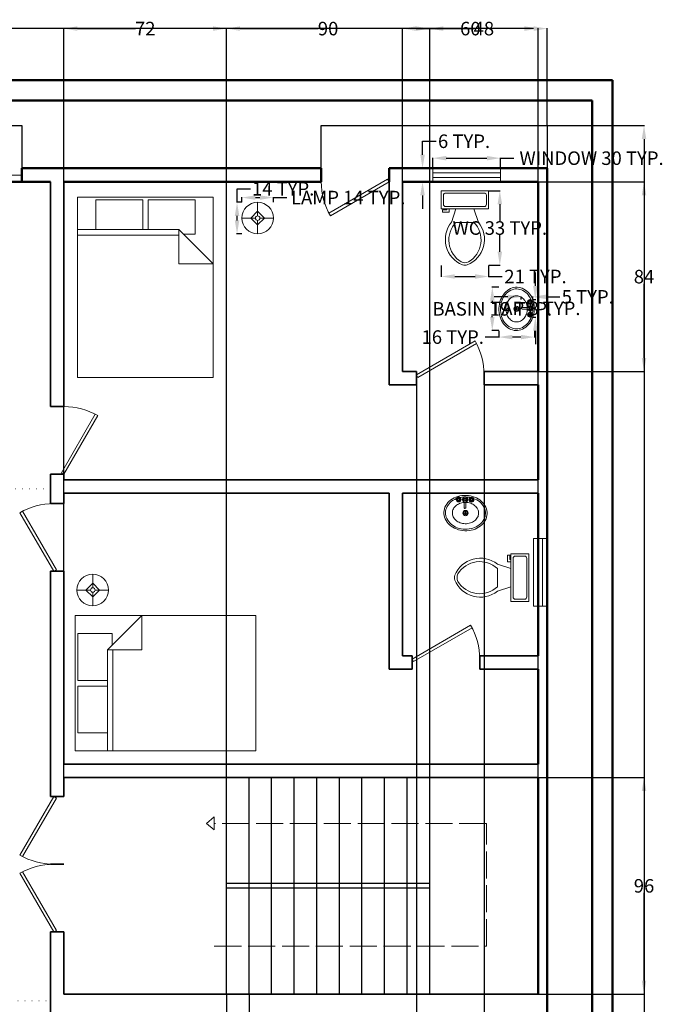
# Model space of a CAD drawing. Units: inches. Extents: x 910 to 1553, y 598 to 1516.
# Tile 6 of 6: x 1268 to 1553, y 1079 to 1516. Entities that reach past the tile are written whole.
import ezdxf

# ---------------------------------------------------------------- set-up
doc = ezdxf.new("R2010")
doc.units = ezdxf.units.IN
doc.header["$MEASUREMENT"] = 0
doc.linetypes.add('ACAD_ISO02W100', pattern=[15, 12, -3])
doc.linetypes.add('ACAD_ISO07W100', pattern=[3, 0, -3])
for name, color, linetype, lineweight in [('A-ANNO-DIMS', 2, 'Continuous', 18), ('A-ANNO-SYMB', 7, 'Continuous', 13), ('A-FLOR-BALC', 8, 'Continuous', 25), ('A-FLOR-OVHD', 8, 'ACAD_ISO07W100', 13), ('A-FLOR-STRS', 7, 'Continuous', 25), ('A-FLOR-STRS-PATH', 7, 'ACAD_ISO02W100', 13), ('doors', 2, 'Continuous', 18), ('furniture', 11, 'Continuous', 18), ('Inner wall', 230, 'Continuous', 35), ('outer wall', 231, 'Continuous', 50), ('sanitory', 141, 'Continuous', 18), ('windows', 6, 'Continuous', 18)]:
    doc.layers.add(name, color=color, linetype=linetype, lineweight=lineweight)
doc.styles.get("Standard").update_dxf_attribs({"font": 'arial.ttf'})
doc.dimstyles.get("Standard").update_dxf_attribs({"dimtxt": 6, "dimasz": 6, "dimexe": 0.18, "dimexo": 0.0625, "dimgap": 0.09, "dimtad": 0, "dimtih": 1, "dimtoh": 1, "dimdec": 0, "dimzin": 0, "dimdsep": 46, "dimlunit": 3, "dimtxsty": 'Standard', "dimcen": 0.09, "dimadec": 0, "dimazin": 0, "dimtfac": 1, "dimtdec": 0, "dimtofl": 0, "dimtmove": 0, "dimatfit": 3, "dimfxl": 1, "dimtolj": 1, "dimtzin": 0, "dimarcsym": 0})

# ---------------------------------------------------------------- blocks, each defined once
blk = doc.blocks.new('*U2')
for p, q in [((0, 0), (0, -6)), ((40, 0), (40, -6))]:
    blk.add_line(p, q)
blk.add_lwpolyline([(0, 0), (34.64, 20), (35.52, 18.48), (0.87, -1.52)], close=True)
blk.add_arc((0, 0), 40, 0, 30)
blk = doc.blocks.new('*U4')
for p, q in [((0, 0), (0, 6)), ((40, 0), (40, 6))]:
    blk.add_line(p, q)
blk.add_lwpolyline([(0, 0), (34.64, -20), (35.52, -18.48), (0.87, 1.52)], close=True)
blk.add_arc((0, 0), 40, 330, 0)
blk = doc.blocks.new('*U5')
for p, q in [((0, 0), (0, -6)), ((-40, 0), (-40, -6))]:
    blk.add_line(p, q)
blk.add_lwpolyline([(0, 0), (-34.64, 20), (-35.52, 18.48), (-0.88, -1.52)], close=True)
blk.add_arc((0, 0), 40, 150, 180)
blk = doc.blocks.new('*U7')
for p, q in [((-40, 0), (-40, 6)), ((0, 0), (0, 6))]:
    blk.add_line(p, q)
blk.add_lwpolyline([(0, 0), (-34.64, -20), (-35.52, -18.48), (-0.88, 1.52)], close=True)
blk.add_arc((0, 0), 40, 180, 210)
blk = doc.blocks.new('Bed - Queen')
for p, q in [((0, -80.00003), (0, 0)), ((0, 0), (59.99999, 0)), ((59.99999, 0), (59.99999, -80.00003)), ((7.99999, -1.2), (28.79998, -1.2)), ((7.99999, -14.4), (7.99999, -1.2)), ((28.79998, -1.2), (28.79998, -14.4)), ((31.19999, -1.2), (51.99999, -1.2)), ((31.19999, -14.4), (31.19999, -1.2)), ((51.99999, -1.2), (51.99999, -16.4)), ((0, -14.4), (44.8, -14.4)), ((44.8, -16.8), (0, -16.8)), ((59.99999, -29.6), (44.8, -14.4)), ((44.8, -14.4), (44.8, -29.6)), ((51.99999, -16.4), (46.79936, -16.4)), ((44.8, -29.6), (59.99999, -29.6)), ((59.99999, -80.00003), (0, -80.00003))]:
    blk.add_line(p, q)
blk = doc.blocks.new('Lamp - Table')
for p, q in [((0, 7), (0, 1)), ((-1, 0), (-7, 0)), ((0, 3), (-3, 0)), ((-3, 0), (0, -3)), ((3, 0), (0, 3)), ((0, -3), (3, 0)), ((1, 0), (7, 0)), ((0, -1), (0, -7))]:
    blk.add_line(p, q)
for radius in [7, 1]:
    blk.add_circle((0, 0), radius)
blk = doc.blocks.new('Toilet - top')
for p, q in [((9.5, -6), (9.5, -2)), ((-10, -8.5), (-8, -8.5)), ((-10, -9.5), (-10, -8.5)), ((-8, -8.5), (-8, -8)), ((-7, -8), (-7, -9.5)), ((-4, -8), (-6, -14)), ((4, -8), (6, -14)), ((-7, -9.5), (-10, -9.5)), ((4, -14), (-4, -14))]:
    blk.add_line(p, q)
blk.add_lwpolyline([(10.5, -8), (10.5, 0), (-10.5, 0), (-10.5, -8)], close=True)
for points in [[(-9.5, -2), (-9.5, -6)], [(8.5, -1), (-8.5, -1)], [(-8.5, -7), (8.5, -7)]]:
    blk.add_lwpolyline(points)
for centre, radius, start, end in [((-8.62, -1.88), 0.884, 81.8699, 188.1301), ((8.62, -1.88), 0.884, 351.8699, 98.1301), ((-8.62, -6.12), 0.884, 171.8699, 278.1301), ((8.62, -6.12), 0.884, 261.8699, 8.1301), ((3.52, -21.58), 12.17, 141.4691, 247.9714), ((4.2, -21.82), 11.33, 136.3677, 238.9468), ((-3.52, -21.58), 12.17, 292.0284, 38.5307), ((-4.2, -21.82), 11.33, 301.053, 43.6321), ((0, -27.88), 4, 245.7318, 294.2682), ((0, -29), 4, 254.8605, 285.1395)]:
    blk.add_arc(centre, radius, start, end)
blk = doc.blocks.new('Faucet - Bathroom top')
for p, q in [((-4.107, 0.125), (-4.375, 0.125)), ((-3.75, 0.4788), (-3.75, 0.75)), ((-3.5, 0.482), (-3.5, 0.75)), ((-3.1461, 0.125), (-2.875, 0.125)), ((3.143, 0.125), (2.875, 0.125)), ((3.5, 0.4788), (3.5, 0.75)), ((3.75, 0.482), (3.75, 0.75)), ((4.1039, 0.125), (4.375, 0.125)), ((-4.1039, -0.125), (-4.375, -0.125)), ((-3.75, -0.4821), (-3.75, -0.75)), ((-3.5, -0.4789), (-3.5, -0.75)), ((-3.143, -0.125), (-2.875, -0.125)), ((-0.5, -0.8639), (-0.5, -4.5)), ((0.5, -4.5), (0.5, -0.8631)), ((3.1461, -0.125), (2.875, -0.125)), ((3.5, -0.4821), (3.5, -0.75)), ((3.75, -0.4789), (3.75, -0.75)), ((4.107, -0.125), (4.375, -0.125))]:
    blk.add_line(p, q)
for centre, radius in [((-3.625, 0), 1.375), ((-4.625, 0), 0.2795), ((-3.625, 0), 0.5), ((-3.625, 1), 0.2795), ((-2.625, 0), 0.2795), ((0, 0), 0.5), ((3.625, 0), 1.375), ((2.625, 0), 0.2795), ((3.625, 0), 0.5), ((3.625, 1), 0.2795), ((4.625, 0), 0.2795), ((-3.625, -1), 0.2795), ((3.625, -1), 0.2795)]:
    blk.add_circle(centre, radius)
for centre, radius, start, end in [((-3.625, 0), 1, 105.2407, 164.2093), ((-3.625, 0), 1, 16.44125, 74.07887), ((0, 0), 1.5, 289.6514, 250.3603), ((0, 0), 1, 300.3431, 239.7554), ((3.625, 0), 1, 106.12, 164.0884), ((3.625, 0), 1, 16.23422, 73.90469), ((-3.625, 0), 1, 196.2342, 253.9047), ((-3.625, 0), 1, 286.12, 344.0884), ((0, -4.5), 0.5, 180, 0), ((3.625, 0), 1, 196.4413, 254.0789), ((3.625, 0), 1, 285.2407, 344.2093)]:
    blk.add_arc(centre, radius, start, end)
blk = doc.blocks.new('Sink - Oval top')
for p, q in [((-1, 0), (1, 0)), ((0, 1), (0, -1))]:
    blk.add_line(p, q)
for points in [[(-12.23, 0.39, 0.117634), (-11.46, -3.36, 0.104469), (-8.88, -6.8, 0.090016), (-5.08, -9.07, 0.08192), (-0.32, -10.02, 0.08192), (4.49, -9.38, 0.090016), (8.42, -7.36, 0.104469), (11.22, -4.09, 0.117634), (12.23, -0.39, 0.117634), (11.46, 3.36, 0.104469), (8.88, 6.8, 0.090016), (5.08, 9.07, 0.08192), (0.32, 10.02, 0.08192), (-4.49, 9.38, 0.090016), (-8.42, 7.36, 0.104469), (-11.22, 4.09, 0.117634)], [(-11.29, 0.16, 0.118622), (-10.52, -3.25, 0.104678), (-8.07, -6.36, 0.089562), (-4.54, -8.37, 0.081185), (-0.13, -9.15, 0.081185), (4.3, -8.49, 0.089562), (7.89, -6.58, 0.104678), (10.42, -3.55, 0.118622), (11.29, -0.16, 0.118622), (10.52, 3.25, 0.104678), (8.07, 6.36, 0.089562), (4.54, 8.37, 0.081185), (0.13, 9.15, 0.081185), (-4.3, 8.49, 0.089562), (-7.89, 6.58, 0.104678), (-10.42, 3.55, 0.118622)], [(-7.42, 0.08, 0.118283), (-6.91, -2.17, 0.104607), (-5.29, -4.21, 0.089718), (-2.97, -5.53, 0.081436), (-0.07, -6.04, 0.081436), (2.84, -5.59, 0.089718), (5.2, -4.33, 0.104607), (6.86, -2.32, 0.118283), (7.42, -0.08, 0.118283), (6.91, 2.17, 0.104607), (5.29, 4.21, 0.089718), (2.97, 5.53, 0.081436), (0.07, 6.04, 0.081436), (-2.84, 5.59, 0.089718), (-5.2, 4.33, 0.104607), (-6.86, 2.32, 0.118283)]]:
    blk.add_lwpolyline(points, format="xyb", close=True)
for radius in [1.5, 1]:
    blk.add_circle((0, 0), radius)
blk = doc.blocks.new('WIN-30X6')
for p, q in [((0, 6), (30, 6)), ((0, 0), (0, 6)), ((30, 6), (30, 0)), ((0, 4), (30, 4)), ((30, 2), (0, 2)), ((30, 0), (0, 0))]:
    blk.add_line(p, q)
blk = doc.blocks.new('VERANDA-EDGE-SHALLOW')
for p, q in [((0, 0), (0, 18.99)), ((0, 18.99), (100, 18.99)), ((100, 18.99), (100, 0))]:
    blk.add_line(p, q)
blk = doc.blocks.new('*D23')
at = {"layer": 'A-ANNO-DIMS', "color": 0, "lineweight": -2, "transparency": 16777216}
for p, q in [((1366.48, 1434.97), (1366.48, 1437.19)), ((1372.48, 1437.01), (1374.48, 1437.01)), ((1380.48, 1434.97), (1380.48, 1437.19)), ((1380.48, 1437.01), (1386.48, 1437.01))]:
    blk.add_line(p, q, dxfattribs=at)
for points in [[(1372.48, 1438.01), (1372.48, 1436.01), (1366.48, 1437.01)], [(1374.48, 1438.01), (1374.48, 1436.01), (1380.48, 1437.01)]]:
    blk.add_solid(points, dxfattribs=at)
at = {"layer": 'Defpoints', "color": 0, "lineweight": -2, "transparency": 16777216}
for p in [(1380.48, 1437.01), (1366.48, 1434.91), (1380.48, 1434.91)]:
    blk.add_point(p, dxfattribs=at)
at = {"layer": 'A-ANNO-DIMS', "color": 0, "transparency": 16777216, "insert": (1413.62, 1437.01), "char_height": 6, "attachment_point": 5}
blk.add_mtext('\\A1;LAMP 14 TYP.', dxfattribs=at)
blk = doc.blocks.new('*D24')
at = {"layer": 'A-ANNO-DIMS', "color": 0, "lineweight": -2, "transparency": 16777216}
for p, q in [((1364.38, 1434.91), (1364.38, 1440.91)), ((1364.38, 1440.91), (1370.38, 1440.91)), ((1366.42, 1434.91), (1364.2, 1434.91)), ((1364.38, 1426.91), (1364.38, 1428.91)), ((1366.42, 1420.91), (1364.2, 1420.91))]:
    blk.add_line(p, q, dxfattribs=at)
for points in [[(1363.38, 1428.91), (1365.38, 1428.91), (1364.38, 1434.91)], [(1363.38, 1426.91), (1365.38, 1426.91), (1364.38, 1420.91)]]:
    blk.add_solid(points, dxfattribs=at)
at = {"layer": 'Defpoints', "color": 0, "lineweight": -2, "transparency": 16777216}
for p in [(1364.38, 1434.91), (1366.48, 1434.91), (1366.48, 1420.91)]:
    blk.add_point(p, dxfattribs=at)
at = {"layer": 'A-ANNO-DIMS', "color": 0, "transparency": 16777216, "insert": (1384.79, 1440.91), "char_height": 6, "attachment_point": 5}
blk.add_mtext('\\A1;14 TYP.', dxfattribs=at)
blk = doc.blocks.new('*D29')
at = {"layer": 'A-ANNO-DIMS', "color": 0, "lineweight": -2, "transparency": 16777216}
for p, q in [((1475.88, 1440.03), (1480.95, 1440.03)), ((1480.77, 1434.03), (1480.77, 1426.7)), ((1480.77, 1412.99), (1480.77, 1420.32)), ((1475.88, 1406.99), (1480.95, 1406.99))]:
    blk.add_line(p, q, dxfattribs=at)
for points in [[(1479.77, 1434.03), (1481.77, 1434.03), (1480.77, 1440.03)], [(1479.77, 1412.99), (1481.77, 1412.99), (1480.77, 1406.99)]]:
    blk.add_solid(points, dxfattribs=at)
at = {"layer": 'Defpoints', "color": 0, "lineweight": -2, "transparency": 16777216}
for p in [(1475.81, 1440.03), (1480.77, 1440.03), (1475.81, 1406.99)]:
    blk.add_point(p, dxfattribs=at)
at = {"layer": 'A-ANNO-DIMS', "color": 0, "transparency": 16777216, "insert": (1480.77, 1423.51), "char_height": 6, "attachment_point": 5}
blk.add_mtext('\\A1;WC 33 TYP.', dxfattribs=at)
blk = doc.blocks.new('*D30')
at = {"layer": 'A-ANNO-DIMS', "color": 0, "lineweight": -2, "transparency": 16777216}
for p, q in [((1454.81, 1406.92), (1454.81, 1401.85)), ((1475.81, 1406.92), (1475.81, 1401.85)), ((1460.81, 1402.03), (1469.81, 1402.03)), ((1475.81, 1402.03), (1481.81, 1402.03))]:
    blk.add_line(p, q, dxfattribs=at)
for points in [[(1460.81, 1403.03), (1460.81, 1401.03), (1454.81, 1402.03)], [(1469.81, 1403.03), (1469.81, 1401.03), (1475.81, 1402.03)]]:
    blk.add_solid(points, dxfattribs=at)
at = {"layer": 'Defpoints', "color": 0, "lineweight": -2, "transparency": 16777216}
for p in [(1454.81, 1406.99), (1475.81, 1406.99), (1475.81, 1402.03)]:
    blk.add_point(p, dxfattribs=at)
at = {"layer": 'A-ANNO-DIMS', "color": 0, "transparency": 16777216, "insert": (1496.56, 1402.03), "char_height": 6, "attachment_point": 5}
blk.add_mtext('\\A1;21 TYP.', dxfattribs=at)
blk = doc.blocks.new('*D31')
at = {"layer": 'A-ANNO-DIMS', "color": 0, "lineweight": -2, "transparency": 16777216}
for p, q in [((1480.26, 1397.29), (1477.25, 1397.29)), ((1477.43, 1391.29), (1477.43, 1390.87)), ((1477.43, 1384.06), (1477.43, 1384.48)), ((1480.26, 1378.06), (1477.25, 1378.06))]:
    blk.add_line(p, q, dxfattribs=at)
for points in [[(1476.43, 1391.29), (1478.43, 1391.29), (1477.43, 1397.29)], [(1476.43, 1384.06), (1478.43, 1384.06), (1477.43, 1378.06)]]:
    blk.add_solid(points, dxfattribs=at)
at = {"layer": 'Defpoints', "color": 0, "lineweight": -2, "transparency": 16777216}
for p in [(1477.43, 1397.29), (1480.32, 1397.29), (1480.32, 1378.06)]:
    blk.add_point(p, dxfattribs=at)
at = {"layer": 'A-ANNO-DIMS', "color": 0, "transparency": 16777216, "insert": (1477.43, 1387.68), "char_height": 6, "attachment_point": 5}
blk.add_mtext('\\A1;BASIN 19 TYP.', dxfattribs=at)
blk = doc.blocks.new('*D32')
at = {"layer": 'A-ANNO-DIMS', "color": 0, "lineweight": -2, "transparency": 16777216}
for p, q in [((1480.32, 1375.18), (1474.32, 1375.18)), ((1480.32, 1378), (1480.32, 1375)), ((1490.09, 1375.18), (1486.32, 1375.18)), ((1496.09, 1378), (1496.09, 1375))]:
    blk.add_line(p, q, dxfattribs=at)
for points in [[(1486.32, 1376.18), (1486.32, 1374.18), (1480.32, 1375.18)], [(1490.09, 1376.18), (1490.09, 1374.18), (1496.09, 1375.18)]]:
    blk.add_solid(points, dxfattribs=at)
at = {"layer": 'Defpoints', "color": 0, "lineweight": -2, "transparency": 16777216}
for p in [(1480.32, 1378.06), (1480.32, 1375.18), (1496.09, 1378.06)]:
    blk.add_point(p, dxfattribs=at)
at = {"layer": 'A-ANNO-DIMS', "color": 0, "transparency": 16777216, "insert": (1459.91, 1375.18), "char_height": 6, "attachment_point": 5}
blk.add_mtext('\\A1;16 TYP.', dxfattribs=at)
blk = doc.blocks.new('*D35')
at = {"layer": 'A-ANNO-DIMS', "color": 0, "lineweight": -2, "transparency": 16777216}
for p, q in [((1496.52, 1397.84), (1496.52, 1403.84)), ((1495.41, 1391.84), (1496.7, 1391.84)), ((1495.41, 1384), (1496.7, 1384)), ((1496.52, 1378), (1496.52, 1372))]:
    blk.add_line(p, q, dxfattribs=at)
for points in [[(1495.52, 1397.84), (1497.52, 1397.84), (1496.52, 1391.84)], [(1495.52, 1378), (1497.52, 1378), (1496.52, 1384)]]:
    blk.add_solid(points, dxfattribs=at)
at = {"layer": 'Defpoints', "color": 0, "lineweight": -2, "transparency": 16777216}
for p in [(1495.35, 1391.84), (1495.35, 1384), (1496.52, 1384)]:
    blk.add_point(p, dxfattribs=at)
at = {"layer": 'A-ANNO-DIMS', "color": 0, "transparency": 16777216, "insert": (1496.52, 1387.92), "char_height": 6, "attachment_point": 5}
blk.add_mtext('\\A1;TAP 8 TYP.', dxfattribs=at)
blk = doc.blocks.new('*D36')
at = {"layer": 'A-ANNO-DIMS', "color": 0, "lineweight": -2, "transparency": 16777216}
for p, q in [((1484.26, 1393.01), (1478.26, 1393.01)), ((1490.26, 1391.9), (1490.26, 1393.19)), ((1495.35, 1391.9), (1495.35, 1393.19)), ((1501.35, 1393.01), (1507.35, 1393.01))]:
    blk.add_line(p, q, dxfattribs=at)
for points in [[(1484.26, 1394.01), (1484.26, 1392.01), (1490.26, 1393.01)], [(1501.35, 1394.01), (1501.35, 1392.01), (1495.35, 1393.01)]]:
    blk.add_solid(points, dxfattribs=at)
at = {"layer": 'Defpoints', "color": 0, "lineweight": -2, "transparency": 16777216}
for p in [(1495.35, 1393.01), (1490.26, 1391.84), (1495.35, 1391.84)]:
    blk.add_point(p, dxfattribs=at)
at = {"layer": 'A-ANNO-DIMS', "color": 0, "transparency": 16777216, "insert": (1519.71, 1393.01), "char_height": 6, "attachment_point": 5}
blk.add_mtext('\\A1;5 TYP.', dxfattribs=at)
blk = doc.blocks.new('*D39')
at = {"layer": 'A-ANNO-DIMS', "color": 0, "lineweight": -2, "transparency": 16777216}
for p, q in [((1451.04, 1450.03), (1451.04, 1454.65)), ((1457.04, 1454.47), (1475.04, 1454.47)), ((1481.04, 1450.03), (1481.04, 1454.65)), ((1481.04, 1454.47), (1487.04, 1454.47))]:
    blk.add_line(p, q, dxfattribs=at)
for points in [[(1457.04, 1455.47), (1457.04, 1453.47), (1451.04, 1454.47)], [(1475.04, 1455.47), (1475.04, 1453.47), (1481.04, 1454.47)]]:
    blk.add_solid(points, dxfattribs=at)
at = {"layer": 'Defpoints', "color": 0, "lineweight": -2, "transparency": 16777216}
for p in [(1481.04, 1454.47), (1451.04, 1449.97), (1481.04, 1449.97)]:
    blk.add_point(p, dxfattribs=at)
at = {"layer": 'A-ANNO-DIMS', "color": 0, "transparency": 16777216, "insert": (1521.41, 1454.47), "char_height": 6, "attachment_point": 5}
blk.add_mtext('\\A1;WINDOW 30 TYP.', dxfattribs=at)
blk = doc.blocks.new('*D40')
at = {"layer": 'A-ANNO-DIMS', "color": 0, "lineweight": -2, "transparency": 16777216}
for p, q in [((1446.54, 1455.97), (1446.54, 1461.97)), ((1446.54, 1461.97), (1452.54, 1461.97)), ((1450.98, 1449.97), (1446.36, 1449.97)), ((1450.98, 1443.97), (1446.36, 1443.97)), ((1446.54, 1437.97), (1446.54, 1431.97))]:
    blk.add_line(p, q, dxfattribs=at)
for points in [[(1445.54, 1455.97), (1447.54, 1455.97), (1446.54, 1449.97)], [(1445.54, 1437.97), (1447.54, 1437.97), (1446.54, 1443.97)]]:
    blk.add_solid(points, dxfattribs=at)
at = {"layer": 'Defpoints', "color": 0, "lineweight": -2, "transparency": 16777216}
for p in [(1446.54, 1449.97), (1451.04, 1449.97), (1451.04, 1443.97)]:
    blk.add_point(p, dxfattribs=at)
at = {"layer": 'A-ANNO-DIMS', "color": 0, "transparency": 16777216, "insert": (1464.92, 1461.97), "char_height": 6, "attachment_point": 5}
blk.add_mtext('\\A1;6 TYP.', dxfattribs=at)
blk = doc.blocks.new('*D55')
at = {"layer": 'A-ANNO-DIMS', "color": 0, "lineweight": -2, "transparency": 16777216}
for p, q in [((959.7, 1469.02), (959.7, 1512.08)), ((965.7, 1511.9), (1224.01, 1511.9)), ((1495.7, 1511.9), (1237.39, 1511.9)), ((1501.7, 1469.02), (1501.7, 1512.08))]:
    blk.add_line(p, q, dxfattribs=at)
for points in [[(965.7, 1512.9), (965.7, 1510.9), (959.7, 1511.9)], [(1495.7, 1512.9), (1495.7, 1510.9), (1501.7, 1511.9)]]:
    blk.add_solid(points, dxfattribs=at)
at = {"layer": 'Defpoints', "color": 0, "lineweight": -2, "transparency": 16777216}
for p in [(1501.7, 1511.9), (959.7, 1468.95), (1501.7, 1468.95)]:
    blk.add_point(p, dxfattribs=at)
at = {"layer": 'A-ANNO-DIMS', "color": 0, "transparency": 16777216, "insert": (1230.7, 1511.9), "char_height": 6, "attachment_point": 5}
blk.add_mtext('\\A1;542', dxfattribs=at)
blk = doc.blocks.new('*D56')
at = {"layer": 'A-ANNO-DIMS', "color": 0, "lineweight": -2, "transparency": 16777216}
for p, q in [((1501.76, 1468.95), (1544.83, 1468.95)), ((1544.65, 1462.95), (1544.65, 1060.13)), ((1544.65, 650.99), (1544.65, 1053.82)), ((1501.76, 644.99), (1544.83, 644.99))]:
    blk.add_line(p, q, dxfattribs=at)
for points in [[(1543.65, 1462.95), (1545.65, 1462.95), (1544.65, 1468.95)], [(1543.65, 650.99), (1545.65, 650.99), (1544.65, 644.99)]]:
    blk.add_solid(points, dxfattribs=at)
at = {"layer": 'Defpoints', "color": 0, "lineweight": -2, "transparency": 16777216}
for p in [(1501.7, 1468.95), (1544.65, 1468.95), (1501.7, 644.99)]:
    blk.add_point(p, dxfattribs=at)
at = {"layer": 'A-ANNO-DIMS', "color": 0, "transparency": 16777216, "insert": (1544.65, 1056.97), "char_height": 6, "attachment_point": 5}
blk.add_mtext('\\A1;824', dxfattribs=at)
blk = doc.blocks.new('*D71')
at = {"layer": 'A-ANNO-DIMS', "color": 0, "lineweight": -2, "transparency": 16777216}
for p, q in [((1437.7, 1444.03), (1437.7, 1512.08)), ((1443.7, 1511.9), (1463.31, 1511.9)), ((1491.7, 1511.9), (1472.09, 1511.9)), ((1497.7, 1444.03), (1497.7, 1512.08))]:
    blk.add_line(p, q, dxfattribs=at)
for points in [[(1443.7, 1512.9), (1443.7, 1510.9), (1437.7, 1511.9)], [(1491.7, 1512.9), (1491.7, 1510.9), (1497.7, 1511.9)]]:
    blk.add_solid(points, dxfattribs=at)
at = {"layer": 'Defpoints', "color": 0, "lineweight": -2, "transparency": 16777216}
for p in [(1497.7, 1511.9), (1437.7, 1443.97), (1497.7, 1443.97)]:
    blk.add_point(p, dxfattribs=at)
at = {"layer": 'A-ANNO-DIMS', "color": 0, "transparency": 16777216, "insert": (1467.7, 1511.9), "char_height": 6, "attachment_point": 5}
blk.add_mtext('\\A1;60', dxfattribs=at)
blk = doc.blocks.new('*D72')
at = {"layer": 'A-ANNO-DIMS', "color": 0, "lineweight": -2, "transparency": 16777216}
for p, q in [((1497.76, 1443.97), (1544.83, 1443.97)), ((1544.65, 1437.97), (1544.65, 1405.12)), ((1544.65, 1365.97), (1544.65, 1398.82)), ((1497.76, 1359.97), (1544.83, 1359.97))]:
    blk.add_line(p, q, dxfattribs=at)
for points in [[(1543.65, 1437.97), (1545.65, 1437.97), (1544.65, 1443.97)], [(1543.65, 1365.97), (1545.65, 1365.97), (1544.65, 1359.97)]]:
    blk.add_solid(points, dxfattribs=at)
at = {"layer": 'Defpoints', "color": 0, "lineweight": -2, "transparency": 16777216}
for p in [(1497.7, 1443.97), (1544.65, 1443.97), (1497.7, 1359.97)]:
    blk.add_point(p, dxfattribs=at)
at = {"layer": 'A-ANNO-DIMS', "color": 0, "transparency": 16777216, "insert": (1544.65, 1401.97), "char_height": 6, "attachment_point": 5}
blk.add_mtext('\\A1;84', dxfattribs=at)
blk = doc.blocks.new('*D73')
at = {"layer": 'A-ANNO-DIMS', "color": 0, "lineweight": -2, "transparency": 16777216}
for p, q in [((1443.82, 1359.91), (1443.82, 601.86)), ((1473.82, 1359.91), (1473.82, 601.86)), ((1449.82, 602.04), (1454.45, 602.04)), ((1467.82, 602.04), (1463.2, 602.04))]:
    blk.add_line(p, q, dxfattribs=at)
for points in [[(1449.82, 603.04), (1449.82, 601.04), (1443.82, 602.04)], [(1467.82, 603.04), (1467.82, 601.04), (1473.82, 602.04)]]:
    blk.add_solid(points, dxfattribs=at)
at = {"layer": 'Defpoints', "color": 0, "lineweight": -2, "transparency": 16777216}
for p in [(1443.82, 1359.97), (1473.82, 1359.97), (1473.82, 602.04)]:
    blk.add_point(p, dxfattribs=at)
at = {"layer": 'A-ANNO-DIMS', "color": 0, "transparency": 16777216, "insert": (1458.82, 602.04), "char_height": 6, "attachment_point": 5}
blk.add_mtext('\\A1;30', dxfattribs=at)
blk = doc.blocks.new('*D77')
at = {"layer": 'A-ANNO-DIMS', "color": 0, "lineweight": -2, "transparency": 16777216}
for p, q in [((1287.7, 1180.03), (1287.7, 1512.08)), ((1293.7, 1511.9), (1319.37, 1511.9)), ((1353.7, 1511.9), (1328.03, 1511.9)), ((1359.7, 1180.03), (1359.7, 1512.08))]:
    blk.add_line(p, q, dxfattribs=at)
for points in [[(1293.7, 1512.9), (1293.7, 1510.9), (1287.7, 1511.9)], [(1353.7, 1512.9), (1353.7, 1510.9), (1359.7, 1511.9)]]:
    blk.add_solid(points, dxfattribs=at)
at = {"layer": 'Defpoints', "color": 0, "lineweight": -2, "transparency": 16777216}
for p in [(1359.7, 1511.9), (1287.7, 1179.97), (1359.7, 1179.97)]:
    blk.add_point(p, dxfattribs=at)
at = {"layer": 'A-ANNO-DIMS', "color": 0, "transparency": 16777216, "insert": (1323.7, 1511.9), "char_height": 6, "attachment_point": 5}
blk.add_mtext('\\A1;72', dxfattribs=at)
blk = doc.blocks.new('*D78')
at = {"layer": 'A-ANNO-DIMS', "color": 0, "lineweight": -2, "transparency": 16777216}
for p, q in [((1359.7, 1180.03), (1359.7, 1512.08)), ((1365.7, 1511.9), (1400.32, 1511.9)), ((1443.7, 1511.9), (1409.08, 1511.9)), ((1449.7, 1180.03), (1449.7, 1512.08))]:
    blk.add_line(p, q, dxfattribs=at)
for points in [[(1365.7, 1512.9), (1365.7, 1510.9), (1359.7, 1511.9)], [(1443.7, 1512.9), (1443.7, 1510.9), (1449.7, 1511.9)]]:
    blk.add_solid(points, dxfattribs=at)
at = {"layer": 'Defpoints', "color": 0, "lineweight": -2, "transparency": 16777216}
for p in [(1449.7, 1511.9), (1359.7, 1179.97), (1449.7, 1179.97)]:
    blk.add_point(p, dxfattribs=at)
at = {"layer": 'A-ANNO-DIMS', "color": 0, "transparency": 16777216, "insert": (1404.7, 1511.9), "char_height": 6, "attachment_point": 5}
blk.add_mtext('\\A1;90', dxfattribs=at)
blk = doc.blocks.new('*D79')
at = {"layer": 'A-ANNO-DIMS', "color": 0, "lineweight": -2, "transparency": 16777216}
for p, q in [((1449.7, 1180.03), (1449.7, 1512.08)), ((1455.7, 1511.9), (1469.19, 1511.9)), ((1491.7, 1511.9), (1478.21, 1511.9)), ((1497.7, 1180.03), (1497.7, 1512.08))]:
    blk.add_line(p, q, dxfattribs=at)
for points in [[(1455.7, 1512.9), (1455.7, 1510.9), (1449.7, 1511.9)], [(1491.7, 1512.9), (1491.7, 1510.9), (1497.7, 1511.9)]]:
    blk.add_solid(points, dxfattribs=at)
at = {"layer": 'Defpoints', "color": 0, "lineweight": -2, "transparency": 16777216}
for p in [(1497.7, 1511.9), (1449.7, 1179.97), (1497.7, 1179.97)]:
    blk.add_point(p, dxfattribs=at)
at = {"layer": 'A-ANNO-DIMS', "color": 0, "transparency": 16777216, "insert": (1473.7, 1511.9), "char_height": 6, "attachment_point": 5}
blk.add_mtext('\\A1;48', dxfattribs=at)
blk = doc.blocks.new('*D80')
at = {"layer": 'A-ANNO-DIMS', "color": 0, "lineweight": -2, "transparency": 16777216}
for p, q in [((1497.76, 1179.97), (1544.83, 1179.97)), ((1544.65, 1173.97), (1544.65, 1135.12)), ((1544.65, 1089.97), (1544.65, 1128.82)), ((1497.76, 1083.97), (1544.83, 1083.97))]:
    blk.add_line(p, q, dxfattribs=at)
for points in [[(1543.65, 1173.97), (1545.65, 1173.97), (1544.65, 1179.97)], [(1543.65, 1089.97), (1545.65, 1089.97), (1544.65, 1083.97)]]:
    blk.add_solid(points, dxfattribs=at)
at = {"layer": 'Defpoints', "color": 0, "lineweight": -2, "transparency": 16777216}
for p in [(1497.7, 1179.97), (1544.65, 1179.97), (1497.7, 1083.97)]:
    blk.add_point(p, dxfattribs=at)
at = {"layer": 'A-ANNO-DIMS', "color": 0, "transparency": 16777216, "insert": (1544.65, 1131.97), "char_height": 6, "attachment_point": 5}
blk.add_mtext('\\A1;96', dxfattribs=at)
blk = doc.blocks.new('*D81')
at = {"layer": 'A-ANNO-DIMS', "color": 0, "lineweight": -2, "transparency": 16777216}
for p, q in [((1359.700482, 1083.906924), (1359.700482, 601.863289)), ((1369.700482, 1083.906924), (1369.700482, 601.863289)), ((1353.700482, 602.043289), (1347.700482, 602.043289)), ((1375.700482, 602.043289), (1381.700482, 602.043289))]:
    blk.add_line(p, q, dxfattribs=at)
for points in [[(1353.700482, 603.043289), (1353.700482, 601.043289), (1359.700482, 602.043289)], [(1375.700482, 603.043289), (1375.700482, 601.043289), (1369.700482, 602.043289)]]:
    blk.add_solid(points, dxfattribs=at)
at = {"layer": 'Defpoints', "color": 0, "lineweight": -2, "transparency": 16777216}
for p in [(1359.700482, 1083.969424), (1369.700482, 1083.969424), (1369.700482, 602.043289)]:
    blk.add_point(p, dxfattribs=at)
at = {"layer": 'A-ANNO-DIMS', "color": 0, "transparency": 16777216, "insert": (1364.700482, 602.043289), "char_height": 6, "attachment_point": 5}
blk.add_mtext('\\A1;10', dxfattribs=at)

msp = doc.modelspace()

# ---------------------------------------------------------------- linework, layer by layer
at = {"layer": 'A-ANNO-SYMB'}
for p, q in [((1354.294, 1162.513), (1350.874, 1159.625)), ((1354.294, 1159.625), (1354.294, 1162.513)), ((1354.294, 1156.737), (1350.874, 1159.625)), ((1354.294, 1159.625), (1354.294, 1156.737))]:
    msp.add_line(p, q, dxfattribs=at)
at = {"layer": 'A-FLOR-OVHD'}
for p, q in [((1281.7, 1307.89), (1155.7, 1307.89)), ((1155.7, 1080.969), (1281.7, 1080.969))]:
    msp.add_line(p, q, dxfattribs=at)
at = {"layer": 'A-FLOR-STRS'}
for p, q in [((1359.7, 1083.969), (1359.7, 1179.969)), ((1369.7, 1083.969), (1369.7, 1179.969)), ((1379.7, 1083.969), (1379.7, 1179.969)), ((1389.7, 1083.969), (1389.7, 1179.969)), ((1399.7, 1083.969), (1399.7, 1179.969)), ((1409.7, 1083.969), (1409.7, 1179.969)), ((1419.7, 1083.969), (1419.7, 1179.969)), ((1429.7, 1083.969), (1429.7, 1179.969)), ((1439.7, 1083.969), (1439.7, 1179.969)), ((1449.7, 1083.969), (1449.7, 1179.969)), ((1449.7, 1132.969), (1359.7, 1132.969)), ((1449.7, 1130.969), (1359.7, 1130.969))]:
    msp.add_line(p, q, dxfattribs=at)
at = {"layer": 'A-FLOR-STRS-PATH'}
for p, q in [((1474.817, 1159.625), (1354.294, 1159.625)), ((1474.817, 1105.263), (1474.817, 1159.625)), ((1354.294, 1105.263), (1474.817, 1105.263))]:
    msp.add_line(p, q, dxfattribs=at)
at = {"layer": 'doors'}
for p, q in [((1219.066, 1446.969), (1269.066, 1446.969)), ((1269.066, 1443.969), (1219.066, 1443.969))]:
    msp.add_line(p, q, dxfattribs=at)
at = {"layer": 'Inner wall'}
for p, q in [((1281.7, 1344.4), (1281.7, 1443.969)), ((1287.7, 1344.4), (1287.7, 1443.969)), ((1431.7, 1353.969), (1431.7, 1443.969)), ((1437.7, 1359.969), (1437.7, 1443.969)), ((1437.7, 1359.969), (1443.82, 1359.969)), ((1473.82, 1359.969), (1497.7, 1359.969)), ((1437.7, 1353.969), (1431.7, 1353.969)), ((1437.7, 1353.969), (1443.82, 1353.969)), ((1473.82, 1353.969), (1497.7, 1353.969)), ((1281.7, 1301.379), (1281.7, 1314.4)), ((1287.7, 1311.969), (1287.7, 1314.4)), ((1497.7, 1311.969), (1287.7, 1311.969)), ((1281.7, 1305.969), (1281.7, 1301.379)), ((1287.7, 1305.969), (1287.7, 1301.379)), ((1431.7, 1305.969), (1287.7, 1305.969)), ((1431.7, 1227.969), (1431.7, 1305.969)), ((1497.7, 1305.969), (1437.7, 1305.969)), ((1437.7, 1233.969), (1437.7, 1305.969)), ((1281.7, 1271.379), (1281.7, 1171.545)), ((1287.7, 1271.379), (1287.7, 1185.969)), ((1437.7, 1233.969), (1441.869, 1233.969)), ((1471.869, 1233.969), (1497.7, 1233.969)), ((1437.7, 1227.969), (1431.7, 1227.969)), ((1437.7, 1227.969), (1441.869, 1227.969)), ((1471.869, 1227.969), (1497.7, 1227.969)), ((1497.7, 1185.969), (1287.7, 1185.969)), ((1281.7, 1179.969), (1281.7, 1171.545)), ((1497.7, 1179.969), (1287.7, 1179.969)), ((1287.7, 1179.969), (1287.7, 1171.545)), ((1281.7, 1111.545), (1281.7, 1083.969)), ((1281.7, 1111.545), (1281.7, 1055.242)), ((1287.7, 1111.545), (1287.7, 1083.969)), ((1497.7, 1083.969), (1287.7, 1083.969))]:
    msp.add_line(p, q, dxfattribs=at)
for points in [[(1443.82, 1353.969), (1443.82, 1359.969)], [(1473.82, 1359.969), (1473.82, 1353.969)], [(1281.7, 1344.4), (1287.7, 1344.4)], [(1287.7, 1314.4), (1281.7, 1314.4)], [(1281.7, 1301.379), (1287.7, 1301.379)], [(1287.7, 1271.379), (1281.7, 1271.379)], [(1441.869, 1227.969), (1441.869, 1233.969)], [(1471.869, 1233.969), (1471.869, 1227.969)], [(1281.7, 1171.545), (1287.7, 1171.545)], [(1287.7, 1141.545), (1281.7, 1141.545)], [(1281.7, 1141.545), (1287.7, 1141.545)], [(1287.7, 1111.545), (1281.7, 1111.545)]]:
    msp.add_lwpolyline(points, dxfattribs=at)
at = {"layer": 'outer wall'}
for p, q in [((1521.7, 1479.969), (939.7, 1479.969)), ((1521.7, 633.969), (1521.7, 1479.969)), ((1401.7, 1449.969), (1269.066, 1449.969)), ((1401.7, 1449.969), (1269.066, 1449.969)), ((1269.066, 1449.969), (1269.066, 1443.969)), ((1497.7, 1449.969), (1431.7, 1449.969)), ((1501.7, 1449.969), (1431.7, 1449.969)), ((1497.7, 1449.969), (1501.7, 1449.969)), ((1501.7, 681.969), (1501.7, 1449.969)), ((1281.7, 1443.969), (1219.066, 1443.969)), ((1401.7, 1443.969), (1287.7, 1443.969)), ((1497.7, 1443.969), (1437.7, 1443.969)), ((1497.7, 1359.969), (1497.7, 1443.969)), ((1497.7, 1311.969), (1497.7, 1353.969)), ((1497.7, 1233.969), (1497.7, 1305.969)), ((1497.7, 1185.969), (1497.7, 1227.969)), ((1497.7, 1083.969), (1497.7, 1179.969))]:
    msp.add_line(p, q, dxfattribs=at)
msp.add_lwpolyline([(1530.7, 1488.969), (930.7, 1488.969), (930.7, 624.969), (1530.7, 624.969)], close=True, dxfattribs=at)
for points in [[(1401.7, 1443.969), (1401.7, 1449.969)], [(1431.7, 1449.969), (1431.7, 1443.969)]]:
    msp.add_lwpolyline(points, dxfattribs=at)

# ---------------------------------------------------------------- block references
at = {"layer": 'A-FLOR-BALC'}
for p in [(1169.066, 1449.969), (1401.7, 1449.969)]:
    msp.add_blockref('VERANDA-EDGE-SHALLOW', p, dxfattribs=at)
at = {"layer": 'doors', "xscale": 0.75, "yscale": 0.75, "zscale": 0.75}
for name, p in [('*U7', (1431.7, 1443.969)), ('*U2', (1443.82, 1358.469)), ('*U2', (1441.869, 1232.469))]:
    msp.add_blockref(name, p, dxfattribs=at)
at = {"layer": 'doors', "xscale": 0.75, "yscale": 0.75, "zscale": 0.75, "rotation": 90}
for name, p in [('*U4', (1287.7, 1314.4)), ('*U2', (1283.2, 1271.379)), ('*U5', (1283.2, 1171.545)), ('*U2', (1283.2, 1111.545))]:
    msp.add_blockref(name, p, dxfattribs=at)
at = {"layer": 'furniture'}
for name, p in [('Bed - Queen', (1293.772, 1437.201)), ('Lamp - Table', (1373.484, 1427.909))]:
    msp.add_blockref(name, p, dxfattribs=at)
at = {"layer": 'furniture', "rotation": 90}
for name, p in [('Lamp - Table', (1300.462, 1263.067)), ('Bed - Queen', (1292.623, 1191.738))]:
    msp.add_blockref(name, p, dxfattribs=at)
at = {"layer": 'sanitory'}
msp.add_blockref('Toilet - top', (1465.313, 1440.033), dxfattribs=at)
at = {"layer": 'sanitory', "xscale": 0.7833329843755676, "yscale": 0.7833329843755676, "zscale": 0.7833329843755676}
for name, p, rotation in [('Sink - Oval top', (1488.205, 1387.676), 90), ('Faucet - Bathroom top', (1494.172, 1387.919), 270), ('Sink - Oval top', (1465.56, 1297.189), 179.4453902364626), ('Faucet - Bathroom top', (1465.374, 1303.158), 359.4453902364627)]:
    msp.add_blockref(name, p, dxfattribs=dict(at, rotation=rotation))
at = {"layer": 'sanitory', "rotation": 270}
msp.add_blockref('Toilet - top', (1493.687, 1268.553), dxfattribs=at)
at = {"layer": 'windows'}
msp.add_blockref('WIN-30X6', (1451.039, 1443.969), dxfattribs=at)
at = {"layer": 'windows', "rotation": 90.00000000000033}
msp.add_blockref('WIN-30X6', (1501.7, 1255.89), dxfattribs=at)

# ---------------------------------------------------------------- dimensions: what is measured, and where the dimension line sits
at = {"layer": 'A-ANNO-DIMS'}
for base, p1, p2, picture, middle in [((1501.7, 1511.905), (959.7, 1468.955), (1501.7, 1468.955), '*D55', (1230.7, 1511.905)), ((1359.7, 1511.905), (1287.7, 1179.969), (1359.7, 1179.969), '*D77', (1323.7, 1511.905)), ((1449.7, 1511.905), (1359.7, 1179.969), (1449.7, 1179.969), '*D78', (1404.7, 1511.905)), ((1497.7, 1511.905), (1437.7, 1443.969), (1497.7, 1443.969), '*D71', (1467.7, 1511.905)), ((1497.7, 1511.905), (1449.7, 1179.969), (1497.7, 1179.969), '*D79', (1473.7, 1511.905)), ((1473.82, 602.043), (1443.82, 1359.969), (1473.82, 1359.969), '*D73', (1458.82, 602.043)), ((1369.7, 602.043), (1359.7, 1083.969), (1369.7, 1083.969), '*D81', (1364.7, 602.043))]:
    dim = msp.add_linear_dim(base=base, p1=p1, p2=p2, dimstyle='Standard', override={"dimdec": 0, "dimlfac": 1, "dimrnd": 0, "dimzin": 0, "dimdsep": 46, "dimlunit": 2}, dxfattribs=at)
    dim.commit()
    dim.dimension.update_dxf_attribs({"geometry": picture, "text_midpoint": middle})
for base, p1, p2, angle, text, picture, middle in [((1446.539, 1449.969), (1451.039, 1443.969), (1451.039, 1449.969), 90, '<> TYP.', '*D40', (1464.918, 1461.969)), ((1364.384, 1434.909), (1366.484, 1420.909), (1366.484, 1434.909), 90, '<> TYP.', '*D24', (1384.795, 1440.909)), ((1480.769, 1440.033), (1475.813, 1406.987), (1475.813, 1440.033), 90, 'WC <> TYP.', '*D29', (1480.769, 1423.51)), ((1477.433, 1397.292), (1480.318, 1378.06), (1480.318, 1397.292), 90, 'BASIN <> TYP.', '*D31', (1477.433, 1387.676)), ((1496.522, 1384.002), (1495.347, 1391.836), (1495.347, 1384.002), 270, 'TAP <> TYP.', '*D35', (1496.522, 1387.919)), ((1480.318, 1375.175), (1496.092, 1378.06), (1480.318, 1378.06), 180, '<> TYP.', '*D32', (1459.907, 1375.175))]:
    dim = msp.add_linear_dim(base=base, p1=p1, p2=p2, angle=angle, text=text, dimstyle='Standard', override={"dimdec": 0, "dimlfac": 1, "dimrnd": 0, "dimzin": 0, "dimdsep": 46, "dimlunit": 2}, dxfattribs=at)
    dim.commit()
    dim.dimension.update_dxf_attribs({"geometry": picture, "text_midpoint": middle})
for base, p1, p2, text, picture, middle in [((1481.039, 1454.469), (1451.039, 1449.969), (1481.039, 1449.969), 'WINDOW <> TYP.', '*D39', (1521.408, 1454.469)), ((1380.484, 1437.009), (1366.484, 1434.909), (1380.484, 1434.909), 'LAMP <> TYP.', '*D23', (1413.621, 1437.009)), ((1475.813, 1402.03), (1454.813, 1406.987), (1475.813, 1406.987), '<> TYP.', '*D30', (1496.557, 1402.03)), ((1495.347, 1393.011), (1490.255, 1391.836), (1495.347, 1391.836), '<> TYP.', '*D36', (1519.709, 1393.011))]:
    dim = msp.add_linear_dim(base=base, p1=p1, p2=p2, text=text, dimstyle='Standard', override={"dimdec": 0, "dimlfac": 1, "dimrnd": 0, "dimzin": 0, "dimdsep": 46, "dimlunit": 2}, dxfattribs=at)
    dim.commit()
    dim.dimension.update_dxf_attribs({"geometry": picture, "text_midpoint": middle})
for base, p1, p2, picture, middle in [((1544.65, 1468.955), (1501.7, 644.993), (1501.7, 1468.955), '*D56', (1544.65, 1056.974)), ((1544.65, 1443.969), (1497.7, 1359.969), (1497.7, 1443.969), '*D72', (1544.65, 1401.969)), ((1544.65, 1179.969), (1497.7, 1083.969), (1497.7, 1179.969), '*D80', (1544.65, 1131.969))]:
    dim = msp.add_linear_dim(base=base, p1=p1, p2=p2, angle=90, dimstyle='Standard', override={"dimdec": 0, "dimlfac": 1, "dimrnd": 0, "dimzin": 0, "dimdsep": 46, "dimlunit": 2}, dxfattribs=at)
    dim.commit()
    dim.dimension.update_dxf_attribs({"geometry": picture, "text_midpoint": middle})

doc.saveas('drawing.dxf')
